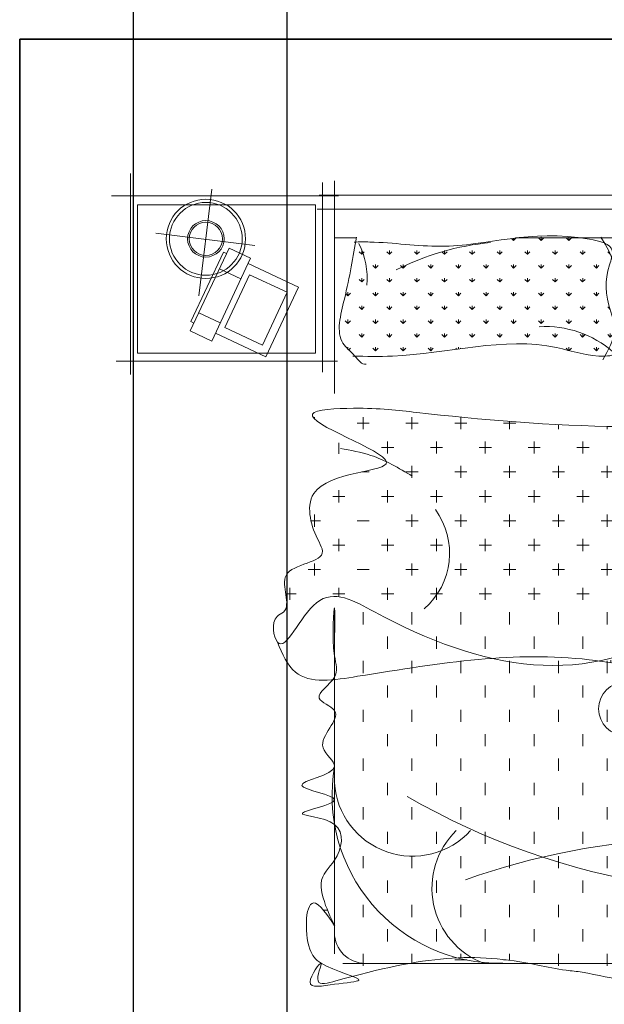
# Model space of a CAD drawing. Units: inches. Extents: x -438 to 102, y -60 to 1091.
# Tile 7 of 20: x -303 to -243, y 699 to 799. Entities that reach past the tile are written whole.
import ezdxf

# ---------------------------------------------------------------- set-up
doc = ezdxf.new("R2010")
doc.units = ezdxf.units.IN
doc.header["$MEASUREMENT"] = 0
doc.layers.add('A-ANNO-DIMS', color=217, linetype='Continuous', lineweight=18, true_color=0x93278f)
doc.layers.add('A-WALL', color=2, linetype='Continuous', lineweight=35, true_color=0xf1eb1f)
doc.layers.add('Furniture', color=7, linetype='Continuous', lineweight=15)
doc.styles.get("Standard").update_dxf_attribs({"font": 'arial.ttf'})
doc.dimstyles.get("Standard").update_dxf_attribs({"dimtxt": 8, "dimasz": 0.18, "dimexe": 0.18, "dimexo": 0.0625, "dimgap": 0.09, "dimtad": 0, "dimtih": 1, "dimtoh": 1, "dimdec": 4, "dimzin": 0, "dimdsep": 46, "dimlunit": 3, "dimtxsty": 'Standard', "dimcen": 0.09, "dimadec": 0, "dimazin": 0, "dimtfac": 1, "dimtdec": 4, "dimtofl": 0, "dimtmove": 0, "dimatfit": 3, "dimfxl": 1, "dimtolj": 1, "dimtzin": 0, "dimarcsym": 0})

# ---------------------------------------------------------------- blocks, each defined once
blk = doc.blocks.new('BED-DOUBLE-WITH-NIGHTSTANDS')
for p, q in [((-50.06, 0), (-50.06, -20.6)), ((30.68, 0), (30.68, -20.6)), ((-30.37, -20.33), (-30.37, -0.9)), ((-29.16, -22.53), (-29.16, -0.74)), ((50.37, -20.33), (50.37, -0.9)), ((-41.72, -1.6), (-43.05, -12.53)), ((29.9, -1.01), (29.9, -27.13)), ((-28.76, -2.28), (-51.98, -2.28)), ((-30.74, -2.19), (29.9, -2.19)), ((51.99, -2.28), (28.76, -2.28)), ((-31.1, -3.21), (-49.32, -3.21)), ((-49.32, -3.21), (-49.32, -18.39)), ((-31.1, -18.39), (-31.1, -3.21)), ((30.68, -3.64), (-30.92, -3.64)), ((49.65, -3.21), (31.43, -3.21)), ((31.43, -3.21), (31.43, -18.39)), ((40.58, -3.96), (40.58, -15.85)), ((49.65, -18.39), (49.65, -3.21)), ((-37.32, -7.35), (-47.47, -6.1)), ((-26.93, -6.59), (-29.16, -6.59)), ((-10.82, -6.85), (-11.02, -6.64)), ((-10.82, -6.85), (-10.55, -6.59)), ((-10.82, -6.85), (-10.82, -6.62)), ((4.24, -6.59), (-10.63, -6.59)), ((-7.99, -6.85), (-8.25, -6.59)), ((-7.99, -6.85), (-7.99, -6.48)), ((-7.99, -6.85), (-7.72, -6.59)), ((-5.16, -6.85), (-5.42, -6.59)), ((-5.16, -6.85), (-5.16, -6.48)), ((-5.16, -6.85), (-4.89, -6.59)), ((5.02, -6.85), (4.75, -6.59)), ((5.02, -6.85), (5.02, -6.53)), ((5.02, -6.85), (5.28, -6.59)), ((29.9, -6.59), (7.41, -6.59)), ((7.85, -6.85), (7.61, -6.61)), ((7.85, -6.85), (7.85, -6.64)), ((7.85, -6.85), (8.03, -6.66)), ((-43.93, -16.11), (-39.96, -7.63)), ((-40.53, -8.03), (-43.86, -15.16)), ((-40.22, -8.18), (-40.53, -8.03)), ((-39.96, -7.63), (-37.75, -8.67)), ((-26.37, -8.26), (-26.64, -8)), ((-26.37, -8.27), (-26.37, -7.89)), ((-26.37, -8.26), (-26.11, -8)), ((-23.54, -8.26), (-23.81, -8)), ((-23.54, -8.27), (-23.54, -7.89)), ((-23.54, -8.26), (-23.28, -8)), ((-20.72, -8.26), (-20.98, -8)), ((-20.72, -8.27), (-20.72, -7.89)), ((-20.72, -8.26), (-20.45, -8)), ((-17.89, -8.26), (-18.15, -8)), ((-17.89, -8.27), (-17.89, -7.89)), ((-17.89, -8.26), (-17.62, -8)), ((-15.06, -8.26), (-15.32, -8)), ((-15.06, -8.27), (-15.06, -7.89)), ((-15.06, -8.26), (-14.79, -8)), ((-12.23, -8.26), (-12.5, -8)), ((-12.23, -8.27), (-12.23, -7.89)), ((-12.23, -8.26), (-11.97, -8)), ((-9.4, -8.26), (-9.67, -8)), ((-9.4, -8.27), (-9.4, -7.89)), ((-9.4, -8.26), (-9.14, -8)), ((-6.57, -8.26), (-6.84, -8)), ((-6.57, -8.27), (-6.57, -7.89)), ((-6.57, -8.26), (-6.31, -8)), ((-3.75, -8.26), (-4.01, -8)), ((-3.75, -8.26), (-3.48, -8)), ((-3.74, -8.27), (-3.74, -7.89)), ((-0.92, -8.26), (-1.18, -8)), ((1.02, -8.02), (1.04, -8)), ((3.6, -8.26), (3.34, -8)), ((3.6, -8.27), (3.6, -7.89)), ((3.6, -8.26), (3.87, -8)), ((6.43, -8.26), (6.17, -8)), ((6.43, -8.27), (6.43, -7.89)), ((6.43, -8.26), (6.7, -8)), ((9.26, -8.26), (9, -8)), ((9.26, -8.27), (9.26, -7.89)), ((9.26, -8.26), (9.53, -8)), ((12.09, -8.26), (11.82, -8)), ((12.09, -8.27), (12.09, -7.89)), ((12.09, -8.26), (12.35, -8)), ((14.92, -8.26), (14.65, -8)), ((14.92, -8.27), (14.92, -7.89)), ((14.92, -8.26), (15.18, -8)), ((17.75, -8.26), (17.48, -8)), ((17.75, -8.27), (17.75, -7.89)), ((17.75, -8.26), (18.01, -8)), ((20.57, -8.26), (20.31, -8)), ((20.57, -8.27), (20.57, -7.89)), ((20.57, -8.26), (20.84, -8)), ((23.4, -8.26), (23.14, -8)), ((23.4, -8.27), (23.4, -7.89)), ((23.4, -8.26), (23.67, -8)), ((26.23, -8.26), (25.97, -8)), ((26.23, -8.27), (26.23, -7.89)), ((26.23, -8.26), (26.5, -8)), ((-37.75, -8.67), (-41.72, -17.15)), ((-0.92, -8.27), (-0.92, -8.26)), ((-0.92, -8.26), (-0.91, -8.26)), ((-38.74, -10.79), (-40.95, -9.75)), ((-32.84, -11.63), (-38.01, -9.21)), ((-24.96, -9.68), (-25.22, -9.41)), ((-24.96, -9.68), (-24.96, -9.3)), ((-24.96, -9.68), (-24.69, -9.41)), ((-22.13, -9.68), (-22.4, -9.41)), ((-22.13, -9.68), (-22.13, -9.3)), ((-22.13, -9.68), (-21.86, -9.41)), ((-19.3, -9.68), (-19.57, -9.41)), ((-19.3, -9.68), (-19.3, -9.3)), ((-19.3, -9.68), (-19.04, -9.41)), ((-16.47, -9.68), (-16.74, -9.41)), ((-16.47, -9.68), (-16.47, -9.3)), ((-16.47, -9.68), (-16.21, -9.41)), ((-13.64, -9.68), (-13.91, -9.41)), ((-13.64, -9.68), (-13.64, -9.3)), ((-13.64, -9.68), (-13.38, -9.41)), ((-10.82, -9.68), (-11.08, -9.41)), ((-10.82, -9.68), (-10.82, -9.3)), ((-10.82, -9.68), (-10.55, -9.41)), ((-7.99, -9.68), (-8.25, -9.41)), ((-7.99, -9.68), (-7.99, -9.3)), ((-7.99, -9.68), (-7.72, -9.41)), ((-5.16, -9.68), (-5.42, -9.41)), ((-5.16, -9.68), (-5.16, -9.3)), ((-5.16, -9.68), (-4.89, -9.41)), ((-2.33, -9.68), (-2.6, -9.41)), ((-2.33, -9.68), (-2.33, -9.3)), ((-2.33, -9.68), (-2.07, -9.41)), ((2.19, -9.68), (1.92, -9.41)), ((2.19, -9.68), (2.19, -9.3)), ((2.19, -9.68), (2.45, -9.41)), ((5.02, -9.68), (4.75, -9.41)), ((5.02, -9.68), (5.02, -9.3)), ((5.02, -9.68), (5.28, -9.41)), ((7.85, -9.68), (7.58, -9.41)), ((7.85, -9.68), (7.85, -9.3)), ((7.85, -9.68), (8.11, -9.41)), ((10.67, -9.68), (10.41, -9.41)), ((10.67, -9.68), (10.94, -9.41)), ((10.68, -9.68), (10.68, -9.3)), ((13.5, -9.68), (13.24, -9.41)), ((13.5, -9.68), (13.5, -9.3)), ((13.5, -9.68), (13.77, -9.41)), ((16.33, -9.68), (16.07, -9.41)), ((16.33, -9.68), (16.33, -9.3)), ((16.33, -9.68), (16.6, -9.41)), ((19.16, -9.68), (18.89, -9.41)), ((19.16, -9.68), (19.16, -9.3)), ((19.16, -9.68), (19.43, -9.41)), ((21.99, -9.68), (21.72, -9.41)), ((21.99, -9.68), (21.99, -9.3)), ((21.99, -9.68), (22.25, -9.41)), ((24.82, -9.68), (24.55, -9.41)), ((24.82, -9.68), (24.82, -9.3)), ((24.82, -9.68), (25.08, -9.41)), ((27.65, -9.68), (27.38, -9.41)), ((27.65, -9.68), (27.65, -9.3)), ((27.65, -9.68), (27.91, -9.41)), ((-37.86, -10.36), (-40.39, -15.77)), ((-34, -12.16), (-37.86, -10.36)), ((-26.37, -11.09), (-26.64, -10.83)), ((-26.37, -11.09), (-26.37, -10.72)), ((-26.37, -11.09), (-26.11, -10.83)), ((-23.54, -11.09), (-23.81, -10.83)), ((-23.54, -11.09), (-23.54, -10.72)), ((-23.54, -11.09), (-23.28, -10.83)), ((-20.72, -11.09), (-20.98, -10.83)), ((-20.72, -11.09), (-20.72, -10.72)), ((-20.72, -11.09), (-20.45, -10.83)), ((-17.89, -11.09), (-18.15, -10.83)), ((-17.89, -11.09), (-17.89, -10.72)), ((-17.89, -11.09), (-17.62, -10.83)), ((-15.06, -11.09), (-15.32, -10.83)), ((-15.06, -11.09), (-15.06, -10.72)), ((-15.06, -11.09), (-14.79, -10.83)), ((-12.23, -11.09), (-12.5, -10.83)), ((-12.23, -11.09), (-12.23, -10.72)), ((-12.23, -11.09), (-11.97, -10.83)), ((-9.4, -11.09), (-9.67, -10.83)), ((-9.4, -11.09), (-9.4, -10.72)), ((-9.4, -11.09), (-9.14, -10.83)), ((-6.57, -11.09), (-6.84, -10.83)), ((-6.57, -11.09), (-6.57, -10.72)), ((-6.57, -11.09), (-6.31, -10.83)), ((-3.75, -11.09), (-4.01, -10.83)), ((-3.75, -11.09), (-3.48, -10.83)), ((-3.74, -11.09), (-3.74, -10.72)), ((3.6, -11.09), (3.34, -10.83)), ((3.6, -11.09), (3.6, -10.72)), ((3.6, -11.09), (3.87, -10.83)), ((6.43, -11.09), (6.17, -10.83)), ((6.43, -11.09), (6.43, -10.72)), ((6.43, -11.09), (6.7, -10.83)), ((9.26, -11.09), (9, -10.83)), ((9.26, -11.09), (9.26, -10.72)), ((9.26, -11.09), (9.53, -10.83)), ((12.09, -11.09), (11.82, -10.83)), ((12.09, -11.09), (12.09, -10.72)), ((12.09, -11.09), (12.35, -10.83)), ((14.92, -11.09), (14.65, -10.83)), ((14.92, -11.09), (14.92, -10.72)), ((14.92, -11.09), (15.18, -10.83)), ((17.75, -11.09), (17.48, -10.83)), ((17.75, -11.09), (17.75, -10.72)), ((17.75, -11.09), (18.01, -10.83)), ((20.57, -11.09), (20.31, -10.83)), ((20.57, -11.09), (20.57, -10.72)), ((20.57, -11.09), (20.84, -10.83)), ((23.4, -11.09), (23.14, -10.83)), ((23.4, -11.09), (23.4, -10.72)), ((23.4, -11.09), (23.67, -10.83)), ((26.23, -11.09), (25.97, -10.83)), ((26.23, -11.09), (26.23, -10.72)), ((26.23, -11.09), (26.5, -10.83)), ((46.48, -10.21), (34.68, -10.21)), ((-36.18, -18.76), (-32.84, -11.63)), ((-36.53, -17.57), (-34, -12.16)), ((-27.79, -12.51), (-28.01, -12.28)), ((-27.79, -12.51), (-27.79, -12.13)), ((-27.79, -12.51), (-27.52, -12.24)), ((-24.96, -12.51), (-25.22, -12.24)), ((-24.96, -12.51), (-24.96, -12.13)), ((-24.96, -12.51), (-24.69, -12.24)), ((-22.13, -12.51), (-22.4, -12.24)), ((-22.13, -12.51), (-22.13, -12.13)), ((-22.13, -12.51), (-21.86, -12.24)), ((-19.3, -12.51), (-19.57, -12.24)), ((-19.3, -12.51), (-19.3, -12.13)), ((-19.3, -12.51), (-19.04, -12.24)), ((-16.47, -12.51), (-16.74, -12.24)), ((-16.47, -12.51), (-16.47, -12.13)), ((-16.47, -12.51), (-16.21, -12.24)), ((-13.64, -12.51), (-13.91, -12.24)), ((-13.64, -12.51), (-13.64, -12.13)), ((-13.64, -12.51), (-13.38, -12.24)), ((-10.82, -12.51), (-11.08, -12.24)), ((-10.82, -12.51), (-10.82, -12.13)), ((-10.82, -12.51), (-10.55, -12.24)), ((-7.99, -12.51), (-8.25, -12.24)), ((-7.99, -12.51), (-7.99, -12.13)), ((-7.99, -12.51), (-7.72, -12.24)), ((-5.16, -12.51), (-5.42, -12.24)), ((-5.16, -12.51), (-5.16, -12.13)), ((-5.16, -12.51), (-4.89, -12.24)), ((-2.33, -12.51), (-2.6, -12.24)), ((-2.33, -12.51), (-2.33, -12.13)), ((-2.33, -12.51), (-2.07, -12.24)), ((2.19, -12.51), (1.92, -12.24)), ((2.19, -12.51), (2.19, -12.13)), ((2.19, -12.51), (2.45, -12.24)), ((5.02, -12.51), (4.75, -12.24)), ((5.02, -12.51), (5.02, -12.13)), ((5.02, -12.51), (5.28, -12.24)), ((7.85, -12.51), (7.58, -12.24)), ((7.85, -12.51), (7.85, -12.13)), ((7.85, -12.51), (8.11, -12.24)), ((10.67, -12.51), (10.41, -12.24)), ((10.67, -12.51), (10.94, -12.24)), ((10.68, -12.51), (10.68, -12.13)), ((13.5, -12.51), (13.24, -12.24)), ((13.5, -12.51), (13.5, -12.13)), ((13.5, -12.51), (13.77, -12.24)), ((16.33, -12.51), (16.07, -12.24)), ((16.33, -12.51), (16.33, -12.13)), ((16.33, -12.51), (16.6, -12.24)), ((19.16, -12.51), (18.89, -12.24)), ((19.16, -12.51), (19.16, -12.13)), ((19.16, -12.51), (19.43, -12.24)), ((21.99, -12.51), (21.72, -12.24)), ((21.99, -12.51), (21.99, -12.13)), ((21.99, -12.51), (22.25, -12.24)), ((24.82, -12.51), (24.55, -12.24)), ((24.82, -12.51), (24.82, -12.13)), ((24.82, -12.51), (25.08, -12.24)), ((27.65, -12.51), (27.38, -12.24)), ((27.65, -12.51), (27.65, -12.13)), ((27.65, -12.51), (27.91, -12.24)), ((-26.37, -13.92), (-26.64, -13.66)), ((-26.37, -13.92), (-26.37, -13.55)), ((-26.37, -13.92), (-26.11, -13.66)), ((-23.54, -13.92), (-23.81, -13.66)), ((-23.54, -13.92), (-23.54, -13.55)), ((-23.54, -13.92), (-23.28, -13.66)), ((-20.72, -13.92), (-20.98, -13.66)), ((-20.72, -13.92), (-20.72, -13.55)), ((-20.72, -13.92), (-20.45, -13.66)), ((-17.89, -13.92), (-18.15, -13.66)), ((-17.89, -13.92), (-17.89, -13.55)), ((-17.89, -13.92), (-17.62, -13.66)), ((-15.06, -13.92), (-15.32, -13.66)), ((-15.06, -13.92), (-15.06, -13.55)), ((-15.06, -13.92), (-14.79, -13.66)), ((-12.23, -13.92), (-12.5, -13.66)), ((-12.23, -13.92), (-12.23, -13.55)), ((-12.23, -13.92), (-11.97, -13.66)), ((-9.4, -13.92), (-9.67, -13.66)), ((-9.4, -13.92), (-9.4, -13.55)), ((-9.4, -13.92), (-9.14, -13.66)), ((-6.57, -13.92), (-6.84, -13.66)), ((-6.57, -13.92), (-6.57, -13.55)), ((-6.57, -13.92), (-6.31, -13.66)), ((-3.75, -13.92), (-4.01, -13.66)), ((-3.75, -13.92), (-3.48, -13.66)), ((-3.74, -13.92), (-3.74, -13.55)), ((-0.93, -13.91), (-1.18, -13.66)), ((1.02, -13.67), (1.04, -13.66)), ((3.6, -13.92), (3.34, -13.66)), ((3.6, -13.92), (3.6, -13.55)), ((3.6, -13.92), (3.87, -13.66)), ((6.43, -13.92), (6.17, -13.66)), ((6.43, -13.92), (6.43, -13.55)), ((6.43, -13.92), (6.7, -13.66)), ((9.26, -13.92), (9, -13.66)), ((9.26, -13.92), (9.26, -13.55)), ((9.26, -13.92), (9.53, -13.66)), ((12.09, -13.92), (11.82, -13.66)), ((12.09, -13.92), (12.09, -13.55)), ((12.09, -13.92), (12.35, -13.66)), ((14.92, -13.92), (14.65, -13.66)), ((14.92, -13.92), (14.92, -13.55)), ((14.92, -13.92), (15.18, -13.66)), ((17.75, -13.92), (17.48, -13.66)), ((17.75, -13.92), (17.75, -13.55)), ((17.75, -13.92), (18.01, -13.66)), ((20.57, -13.92), (20.31, -13.66)), ((20.57, -13.92), (20.57, -13.55)), ((20.57, -13.92), (20.84, -13.66)), ((23.4, -13.92), (23.14, -13.66)), ((23.4, -13.92), (23.4, -13.55)), ((23.4, -13.92), (23.67, -13.66)), ((26.23, -13.92), (25.97, -13.66)), ((26.23, -13.92), (26.23, -13.55)), ((26.23, -13.92), (26.5, -13.66)), ((-40.85, -15.29), (-43.06, -14.25)), ((-27.79, -15.34), (-28.05, -15.07)), ((-27.79, -15.34), (-27.79, -14.96)), ((-27.79, -15.34), (-27.52, -15.07)), ((-24.96, -15.34), (-25.22, -15.07)), ((-24.96, -15.34), (-24.96, -14.96)), ((-24.96, -15.34), (-24.69, -15.07)), ((-22.13, -15.34), (-22.4, -15.07)), ((-22.13, -15.34), (-22.13, -14.96)), ((-22.13, -15.34), (-21.86, -15.07)), ((-19.3, -15.34), (-19.57, -15.07)), ((-19.3, -15.34), (-19.3, -14.96)), ((-19.3, -15.34), (-19.04, -15.07)), ((-16.47, -15.34), (-16.74, -15.07)), ((-16.47, -15.34), (-16.47, -14.96)), ((-16.47, -15.34), (-16.21, -15.07)), ((-13.64, -15.34), (-13.91, -15.07)), ((-13.64, -15.34), (-13.64, -14.96)), ((-13.64, -15.34), (-13.38, -15.07)), ((-10.82, -15.34), (-11.08, -15.07)), ((-10.82, -15.34), (-10.82, -14.96)), ((-10.82, -15.34), (-10.55, -15.07)), ((-7.99, -15.34), (-8.25, -15.07)), ((-7.99, -15.34), (-7.99, -14.96)), ((-7.99, -15.34), (-7.72, -15.07)), ((-5.16, -15.34), (-5.42, -15.07)), ((-5.16, -15.34), (-5.16, -14.96)), ((-5.16, -15.34), (-4.89, -15.07)), ((-2.33, -15.34), (-2.6, -15.07)), ((-2.33, -15.34), (-2.33, -14.96)), ((-2.33, -15.34), (-2.07, -15.07)), ((2.19, -15.34), (1.92, -15.07)), ((2.19, -15.34), (2.19, -14.96)), ((2.19, -15.34), (2.45, -15.07)), ((5.02, -15.34), (4.75, -15.07)), ((5.02, -15.34), (5.02, -14.96)), ((5.02, -15.34), (5.28, -15.07)), ((7.85, -15.34), (7.58, -15.07)), ((7.85, -15.34), (7.85, -14.96)), ((7.85, -15.34), (8.11, -15.07)), ((10.67, -15.34), (10.41, -15.07)), ((10.67, -15.34), (10.94, -15.07)), ((10.68, -15.34), (10.68, -14.96)), ((13.5, -15.34), (13.24, -15.07)), ((13.5, -15.34), (13.5, -14.96)), ((13.5, -15.34), (13.77, -15.07)), ((16.33, -15.34), (16.07, -15.07)), ((16.33, -15.34), (16.33, -14.96)), ((16.33, -15.34), (16.6, -15.07)), ((19.16, -15.34), (18.89, -15.07)), ((19.16, -15.34), (19.16, -14.96)), ((19.16, -15.34), (19.43, -15.07)), ((21.99, -15.34), (21.72, -15.07)), ((21.99, -15.34), (21.99, -14.96)), ((21.99, -15.34), (22.25, -15.07)), ((24.82, -15.34), (24.55, -15.07)), ((24.82, -15.34), (24.82, -14.96)), ((24.82, -15.34), (25.08, -15.07)), ((27.65, -15.34), (27.38, -15.07)), ((27.65, -15.34), (27.65, -14.96)), ((27.65, -15.34), (27.91, -15.07)), ((-41.72, -17.15), (-43.93, -16.11)), ((-43.86, -15.16), (-43.55, -15.31)), ((-40.39, -15.77), (-36.53, -17.57)), ((-41.34, -16.34), (-36.18, -18.76)), ((-26.37, -16.75), (-26.64, -16.48)), ((-26.37, -16.75), (-26.37, -16.38)), ((-26.37, -16.75), (-26.11, -16.48)), ((-23.54, -16.75), (-23.81, -16.48)), ((-23.54, -16.75), (-23.54, -16.38)), ((-23.54, -16.75), (-23.28, -16.48)), ((-20.72, -16.75), (-20.98, -16.48)), ((-20.72, -16.75), (-20.72, -16.38)), ((-20.72, -16.75), (-20.45, -16.48)), ((-17.89, -16.75), (-18.15, -16.48)), ((-17.89, -16.75), (-17.89, -16.38)), ((-17.89, -16.75), (-17.62, -16.48)), ((-15.06, -16.75), (-15.32, -16.48)), ((-15.06, -16.75), (-15.06, -16.38)), ((-15.06, -16.75), (-14.79, -16.48)), ((-12.23, -16.75), (-12.5, -16.48)), ((-12.23, -16.75), (-12.23, -16.38)), ((-12.23, -16.75), (-11.97, -16.48)), ((-9.4, -16.75), (-9.67, -16.48)), ((-9.4, -16.75), (-9.4, -16.38)), ((-9.4, -16.75), (-9.14, -16.48)), ((-6.57, -16.75), (-6.84, -16.48)), ((-6.57, -16.75), (-6.57, -16.38)), ((-6.57, -16.75), (-6.31, -16.48)), ((-3.75, -16.75), (-4.01, -16.48)), ((-3.75, -16.75), (-3.48, -16.48)), ((-3.74, -16.75), (-3.74, -16.38)), ((-0.92, -16.75), (-1.18, -16.48)), ((-0.92, -16.75), (-0.92, -16.38)), ((-0.92, -16.75), (-0.65, -16.48)), ((0.78, -16.75), (0.51, -16.48)), ((0.78, -16.75), (0.78, -16.38)), ((0.78, -16.75), (1.04, -16.48)), ((3.6, -16.75), (3.34, -16.48)), ((3.6, -16.75), (3.6, -16.38)), ((3.6, -16.75), (3.87, -16.48)), ((6.43, -16.75), (6.17, -16.48)), ((6.43, -16.75), (6.43, -16.38)), ((6.43, -16.75), (6.7, -16.48)), ((9.26, -16.75), (9, -16.48)), ((9.26, -16.75), (9.26, -16.38)), ((9.26, -16.75), (9.53, -16.48)), ((12.09, -16.75), (11.82, -16.48)), ((12.09, -16.75), (12.09, -16.38)), ((12.09, -16.75), (12.35, -16.48)), ((14.92, -16.75), (14.65, -16.48)), ((14.92, -16.75), (14.92, -16.38)), ((14.92, -16.75), (15.18, -16.48)), ((17.75, -16.75), (17.48, -16.48)), ((17.75, -16.75), (17.75, -16.38)), ((17.75, -16.75), (18.01, -16.48)), ((20.57, -16.75), (20.31, -16.48)), ((20.57, -16.75), (20.57, -16.38)), ((20.57, -16.75), (20.84, -16.48)), ((23.4, -16.75), (23.14, -16.48)), ((23.4, -16.75), (23.4, -16.38)), ((23.4, -16.75), (23.67, -16.48)), ((26.23, -16.75), (25.97, -16.48)), ((26.23, -16.75), (26.23, -16.38)), ((26.23, -16.75), (26.5, -16.48)), ((29.06, -16.75), (28.79, -16.48)), ((29.06, -16.75), (29.06, -16.38)), ((29.06, -16.75), (29.27, -16.54)), ((-27.79, -17.97), (-27.79, -17.79)), ((-27.69, -18.07), (-27.52, -17.9)), ((-24.96, -18.16), (-25.22, -17.9)), ((-24.96, -18.16), (-24.96, -17.79)), ((-24.96, -18.16), (-24.69, -17.9)), ((-22.13, -18.16), (-22.4, -17.9)), ((-22.13, -18.16), (-22.13, -17.79)), ((-22.13, -18.16), (-21.86, -17.9)), ((-19.3, -18.16), (-19.57, -17.9)), ((-19.3, -18.16), (-19.3, -17.79)), ((-19.3, -18.16), (-19.04, -17.9)), ((-16.65, -17.99), (-16.74, -17.9)), ((-16.47, -17.96), (-16.47, -17.79)), ((-16.24, -17.93), (-16.21, -17.9)), ((-5.21, -18.11), (-5.42, -17.9)), ((-5.16, -18.13), (-5.16, -17.79)), ((-5.13, -18.13), (-4.89, -17.9)), ((-2.33, -18.16), (-2.6, -17.9)), ((-2.33, -18.16), (-2.33, -17.79)), ((-2.33, -18.16), (-2.07, -17.9)), ((2.19, -18.16), (1.92, -17.9)), ((2.19, -18.16), (2.19, -17.79)), ((2.19, -18.16), (2.45, -17.9)), ((5.02, -18.16), (4.75, -17.9)), ((5.02, -18.16), (5.02, -17.79)), ((5.02, -18.16), (5.28, -17.9)), ((7.85, -18.16), (7.58, -17.9)), ((7.85, -18.16), (7.85, -17.79)), ((7.85, -18.16), (8.11, -17.9)), ((10.68, -17.83), (10.68, -17.79)), ((13.5, -17.88), (13.5, -17.79)), ((13.76, -17.91), (13.77, -17.9)), ((16.33, -18.16), (16.07, -17.9)), ((16.33, -18.16), (16.33, -17.79)), ((16.33, -18.16), (16.6, -17.9)), ((19.16, -18.16), (18.89, -17.9)), ((19.16, -18.16), (19.16, -17.79)), ((19.16, -18.16), (19.43, -17.9)), ((21.99, -18.16), (21.72, -17.9)), ((21.99, -18.16), (21.99, -17.79)), ((21.99, -18.16), (22.25, -17.9)), ((24.82, -18.16), (24.55, -17.9)), ((24.82, -18.16), (24.82, -17.79)), ((24.82, -18.16), (25.08, -17.9)), ((27.65, -18.16), (27.38, -17.9)), ((27.65, -18.16), (27.65, -17.79)), ((27.65, -18.16), (27.91, -17.9)), ((30.17, -21.62), (30.17, -17.94)), ((-49.32, -18.39), (-31.1, -18.39)), ((31.43, -18.39), (49.65, -18.39)), ((-51.53, -19.21), (-28.85, -19.21)), ((3.6, -19.24), (3.6, -19.2)), ((29.21, -19.21), (51.9, -19.21)), ((26.28, -23.69), (26.28, -23.21)), ((-31.22, -25.15), (-31.22, -24.94)), ((-26.22, -26.19), (-26.22, -24.94)), ((-21.22, -26.19), (-21.22, -24.94)), ((-16.22, -26.19), (-16.22, -24.95)), ((13.78, -26.19), (13.78, -25.14)), ((18.78, -26.19), (18.78, -24.94)), ((23.78, -26.19), (23.78, -24.94)), ((28.78, -26.19), (28.78, -24.94)), ((-30.59, -25.57), (-30.67, -25.57)), ((-25.59, -25.57), (-26.84, -25.57)), ((-20.59, -25.57), (-21.84, -25.57)), ((-15.59, -25.57), (-16.84, -25.57)), ((-10.59, -25.57), (-11.84, -25.57)), ((-11.22, -26.19), (-11.22, -25.39)), ((-6.22, -26.19), (-6.22, -25.72)), ((-1.22, -26.19), (-1.22, -25.9)), ((3.78, -26.19), (3.78, -25.87)), ((8.78, -26.19), (8.78, -25.62)), ((14.41, -25.57), (13.16, -25.57)), ((19.41, -25.57), (18.16, -25.57)), ((24.41, -25.57), (23.16, -25.57)), ((29.41, -25.57), (28.16, -25.57)), ((-28.71, -28.72), (-28.71, -27.6)), ((-23.09, -28.07), (-24.34, -28.07)), ((-23.72, -28.69), (-23.72, -27.44)), ((-18.09, -28.07), (-19.34, -28.07)), ((-18.72, -28.69), (-18.72, -27.44)), ((-13.09, -28.07), (-14.34, -28.07)), ((-13.72, -28.69), (-13.72, -27.44)), ((-8.09, -28.07), (-9.34, -28.07)), ((-8.72, -28.69), (-8.72, -27.44)), ((-3.09, -28.07), (-4.34, -28.07)), ((-3.72, -28.69), (-3.72, -27.44)), ((1.91, -28.07), (0.66, -28.07)), ((1.28, -28.69), (1.28, -27.44)), ((6.91, -28.07), (5.66, -28.07)), ((6.28, -28.69), (6.28, -27.44)), ((11.91, -28.07), (10.66, -28.07)), ((11.28, -28.69), (11.28, -27.44)), ((16.91, -28.07), (15.66, -28.07)), ((16.28, -28.69), (16.28, -27.44)), ((21.91, -28.07), (20.66, -28.07)), ((21.28, -28.69), (21.28, -27.44)), ((26.91, -28.07), (25.66, -28.07)), ((26.28, -28.69), (26.28, -27.44)), ((31.91, -28.07), (30.66, -28.07)), ((31.28, -28.69), (31.28, -27.44)), ((-21.22, -31.19), (-21.22, -29.94)), ((-16.22, -31.19), (-16.22, -29.94)), ((-11.22, -31.19), (-11.22, -29.94)), ((-6.22, -31.19), (-6.22, -29.94)), ((-1.22, -31.19), (-1.22, -29.94)), ((3.78, -31.19), (3.78, -29.94)), ((8.78, -31.19), (8.78, -29.94)), ((13.78, -31.19), (13.78, -29.94)), ((18.78, -31.19), (18.78, -29.94)), ((23.78, -31.19), (23.78, -29.94)), ((28.78, -31.19), (28.78, -29.94)), ((-25.59, -30.57), (-26.37, -30.57)), ((-20.59, -30.57), (-21.84, -30.57)), ((-15.59, -30.57), (-16.84, -30.57)), ((-10.59, -30.57), (-11.84, -30.57)), ((-5.59, -30.57), (-6.84, -30.57)), ((-0.59, -30.57), (-1.84, -30.57)), ((4.41, -30.57), (3.16, -30.57)), ((9.41, -30.57), (8.16, -30.57)), ((14.41, -30.57), (13.16, -30.57)), ((19.41, -30.57), (18.16, -30.57)), ((24.41, -30.57), (23.16, -30.57)), ((29.41, -30.57), (28.16, -30.57)), ((-28.09, -33.07), (-29.34, -33.07)), ((-28.72, -33.69), (-28.72, -32.44)), ((-23.09, -33.07), (-24.34, -33.07)), ((-23.72, -33.69), (-23.72, -32.44)), ((-18.09, -33.07), (-19.34, -33.07)), ((-18.72, -33.69), (-18.72, -32.44)), ((-13.09, -33.07), (-14.34, -33.07)), ((-13.72, -33.69), (-13.72, -32.44)), ((-8.09, -33.07), (-9.34, -33.07)), ((-8.72, -33.69), (-8.72, -32.44)), ((-3.09, -33.07), (-4.34, -33.07)), ((-3.72, -33.69), (-3.72, -32.44)), ((1.91, -33.07), (0.66, -33.07)), ((1.28, -33.69), (1.28, -32.44)), ((6.91, -33.07), (5.66, -33.07)), ((6.28, -33.69), (6.28, -32.44)), ((11.91, -33.07), (10.66, -33.07)), ((11.28, -33.69), (11.28, -32.44)), ((16.91, -33.07), (15.66, -33.07)), ((16.28, -33.69), (16.28, -32.44)), ((21.91, -33.07), (20.66, -33.07)), ((21.28, -33.69), (21.28, -32.44)), ((26.91, -33.07), (25.66, -33.07)), ((26.28, -33.69), (26.28, -32.44)), ((31.91, -33.07), (30.66, -33.07)), ((31.28, -33.69), (31.28, -32.44)), ((-31.22, -36.19), (-31.22, -34.94)), ((-21.22, -36.19), (-21.22, -34.94)), ((-16.22, -36.19), (-16.22, -34.94)), ((-11.22, -36.19), (-11.22, -34.94)), ((-6.22, -36.19), (-6.22, -34.94)), ((-1.22, -36.19), (-1.22, -34.94)), ((3.78, -36.19), (3.78, -34.94)), ((13.78, -36.19), (13.78, -34.94)), ((18.78, -36.19), (18.78, -34.94)), ((23.78, -36.19), (23.78, -34.94)), ((28.78, -36.19), (28.78, -34.94)), ((-30.59, -35.57), (-31.57, -35.57)), ((-25.59, -35.57), (-26.84, -35.57)), ((-20.59, -35.57), (-21.84, -35.57)), ((-15.59, -35.57), (-16.84, -35.57)), ((-10.59, -35.57), (-11.84, -35.57)), ((-5.59, -35.57), (-6.84, -35.57)), ((-0.59, -35.57), (-1.84, -35.57)), ((4.41, -35.57), (3.16, -35.57)), ((14.41, -35.57), (13.16, -35.57)), ((19.41, -35.57), (18.16, -35.57)), ((24.41, -35.57), (23.16, -35.57)), ((29.41, -35.57), (28.16, -35.57)), ((-28.09, -38.07), (-29.34, -38.07)), ((-28.72, -38.69), (-28.72, -37.44)), ((-23.09, -38.07), (-24.34, -38.07)), ((-23.72, -38.69), (-23.72, -37.44)), ((-18.09, -38.07), (-19.34, -38.07)), ((-18.72, -38.69), (-18.72, -37.44)), ((-13.09, -38.07), (-14.34, -38.07)), ((-13.72, -38.69), (-13.72, -37.44)), ((-8.09, -38.07), (-9.34, -38.07)), ((-8.72, -38.69), (-8.72, -37.44)), ((-3.09, -38.07), (-4.34, -38.07)), ((-3.72, -38.69), (-3.72, -37.44)), ((1.91, -38.07), (0.66, -38.07)), ((1.28, -38.69), (1.28, -37.44)), ((6.91, -38.07), (5.66, -38.07)), ((11.91, -38.07), (10.66, -38.07)), ((11.28, -38.69), (11.28, -37.44)), ((16.91, -38.07), (15.66, -38.07)), ((16.28, -38.69), (16.28, -37.44)), ((21.91, -38.07), (20.66, -38.07)), ((21.28, -38.69), (21.28, -37.44)), ((26.91, -38.07), (25.66, -38.07)), ((26.28, -38.69), (26.28, -37.44)), ((31.91, -38.07), (30.66, -38.07)), ((31.28, -38.69), (31.28, -37.44)), ((-31.22, -41.19), (-31.22, -39.94)), ((-21.22, -41.19), (-21.22, -39.94)), ((-16.22, -41.19), (-16.22, -39.94)), ((-11.22, -41.19), (-11.22, -39.94)), ((-6.22, -41.19), (-6.22, -39.94)), ((-1.22, -41.19), (-1.22, -39.94)), ((3.78, -41.19), (3.78, -39.94)), ((13.78, -41.19), (13.78, -39.94)), ((18.78, -41.19), (18.78, -39.94)), ((23.78, -41.19), (23.78, -39.94)), ((28.78, -41.19), (28.78, -39.94)), ((33.78, -41.19), (33.78, -39.94)), ((-30.59, -40.57), (-31.84, -40.57)), ((-25.59, -40.57), (-26.84, -40.57)), ((-20.59, -40.57), (-21.84, -40.57)), ((-15.59, -40.57), (-16.84, -40.57)), ((-10.59, -40.57), (-11.84, -40.57)), ((-5.59, -40.57), (-6.84, -40.57)), ((-0.59, -40.57), (-1.84, -40.57)), ((4.41, -40.57), (3.16, -40.57)), ((9.41, -40.57), (8.16, -40.57)), ((14.1, -40.57), (13.16, -40.57)), ((20.16, -40.97), (19.43, -40.97)), ((19.79, -41.34), (19.79, -40.86)), ((24.41, -40.57), (24.09, -40.57)), ((29.41, -40.57), (28.16, -40.57)), ((29.9, -41), (29.9, -83.36)), ((34.41, -40.57), (33.16, -40.57)), ((18.32, -42.82), (18.32, -42.08)), ((21.27, -42.82), (21.27, -42.08)), ((24.22, -42.82), (24.22, -42.22)), ((-33.09, -43.07), (-34.15, -43.07)), ((-33.72, -43.69), (-33.72, -42.44)), ((-28.09, -43.07), (-29.34, -43.07)), ((-28.72, -43.37), (-28.72, -42.44)), ((-23.09, -43.07), (-24.34, -43.07)), ((-23.72, -43.69), (-23.72, -42.44)), ((-18.09, -43.07), (-19.34, -43.07)), ((-18.72, -43.69), (-18.72, -42.44)), ((-13.09, -43.07), (-14.34, -43.07)), ((-13.72, -43.69), (-13.72, -42.44)), ((-8.09, -43.07), (-9.34, -43.07)), ((-8.72, -43.69), (-8.72, -42.44)), ((-3.09, -43.07), (-4.34, -43.07)), ((-3.72, -43.69), (-3.72, -42.44)), ((1.91, -43.07), (0.66, -43.07)), ((1.28, -43.69), (1.28, -42.44)), ((6.91, -43.07), (5.66, -43.07)), ((10.92, -43.07), (10.66, -43.07)), ((11.28, -43.69), (11.28, -42.44)), ((15.37, -42.82), (15.37, -42.52)), ((15.73, -42.45), (15.5, -42.45)), ((16.28, -43.69), (16.28, -42.44)), ((18.69, -42.45), (17.95, -42.45)), ((21.64, -42.45), (20.9, -42.45)), ((21.28, -43.69), (21.28, -42.44)), ((24.59, -42.45), (23.85, -42.45)), ((26.28, -43.69), (26.28, -42.44)), ((31.91, -43.07), (30.66, -43.07)), ((31.28, -43.69), (31.28, -42.44)), ((14.26, -43.92), (13.52, -43.92)), ((13.89, -44.29), (13.89, -43.56)), ((17.21, -43.92), (16.47, -43.92)), ((16.84, -44.29), (16.84, -43.56)), ((20.16, -43.92), (19.43, -43.92)), ((19.79, -44.29), (19.79, -43.56)), ((23.12, -43.92), (22.38, -43.92)), ((22.75, -44.29), (22.75, -43.56)), ((26.07, -43.92), (25.33, -43.92)), ((25.7, -44.29), (25.7, -43.56)), ((-29.16, -79.94), (-29.16, -44.49)), ((-26.22, -46.19), (-26.22, -44.94)), ((-21.22, -46.19), (-21.22, -44.94)), ((-16.22, -46.19), (-16.22, -44.94)), ((-11.22, -46.19), (-11.22, -44.94)), ((-6.22, -46.19), (-6.22, -44.94)), ((-1.22, -46.19), (-1.22, -44.94)), ((3.78, -46.19), (3.78, -44.94)), ((8.78, -46.19), (8.78, -44.94)), ((12.78, -45.4), (12.04, -45.4)), ((12.41, -45.77), (12.41, -45.03)), ((13.78, -46.19), (13.78, -44.94)), ((15.73, -45.4), (15, -45.4)), ((15.37, -45.77), (15.37, -45.03)), ((18.69, -45.4), (17.95, -45.4)), ((18.32, -45.77), (18.32, -45.03)), ((18.78, -46.19), (18.78, -44.94)), ((21.64, -45.4), (20.9, -45.4)), ((21.27, -45.77), (21.27, -45.03)), ((23.78, -46.19), (23.78, -44.94)), ((24.47, -45.4), (23.85, -45.4)), ((24.22, -45.56), (24.22, -45.03)), ((28.78, -46.19), (28.78, -44.94)), ((9.41, -45.57), (8.16, -45.57)), ((14.41, -45.57), (13.16, -45.57)), ((19.41, -45.57), (18.16, -45.57)), ((24.41, -45.57), (23.16, -45.57)), ((29.41, -45.57), (28.16, -45.57)), ((7.98, -47.25), (7.98, -47.2)), ((11.31, -46.88), (10.57, -46.88)), ((10.94, -47.25), (10.94, -46.51)), ((14.26, -46.88), (13.52, -46.88)), ((13.89, -47.25), (13.89, -46.51)), ((17.21, -46.88), (16.47, -46.88)), ((16.84, -47.25), (16.84, -46.51)), ((20.16, -46.88), (19.43, -46.88)), ((19.79, -47.25), (19.79, -46.51)), ((22.55, -46.88), (22.38, -46.88)), ((22.75, -46.7), (22.75, -46.51)), ((-34.33, -48.07), (-34.34, -48.07)), ((-23.72, -48.69), (-23.72, -47.44)), ((-18.72, -48.69), (-18.72, -47.44)), ((-13.72, -48.69), (-13.72, -47.44)), ((-8.72, -48.69), (-8.72, -47.44)), ((-3.72, -48.69), (-3.72, -47.44)), ((1.28, -48.69), (1.28, -47.44)), ((6.91, -48.07), (5.66, -48.07)), ((6.88, -48.35), (6.14, -48.35)), ((6.28, -48.69), (6.28, -47.44)), ((6.51, -48.72), (6.51, -47.98)), ((9.83, -48.35), (9.09, -48.35)), ((9.46, -48.72), (9.46, -47.98)), ((11.91, -48.07), (10.66, -48.07)), ((11.28, -48.69), (11.28, -47.44)), ((12.78, -48.35), (12.04, -48.35)), ((12.41, -48.72), (12.41, -47.98)), ((15.73, -48.35), (15, -48.35)), ((15.37, -48.72), (15.37, -47.98)), ((16.91, -48.07), (15.66, -48.07)), ((16.28, -48.69), (16.28, -47.44)), ((18.69, -48.35), (17.95, -48.35)), ((18.32, -48.72), (18.32, -47.98)), ((21.91, -48.07), (20.66, -48.07)), ((21.02, -48.35), (20.9, -48.35)), ((21.27, -48.11), (21.27, -47.98)), ((21.28, -48.69), (21.28, -47.44)), ((26.91, -48.07), (25.66, -48.07)), ((26.28, -48.69), (26.28, -47.44)), ((-26.22, -51.19), (-26.22, -49.94)), ((-21.22, -51.19), (-21.22, -49.94)), ((-16.22, -51.19), (-16.22, -49.94)), ((-11.22, -51.19), (-11.22, -49.94)), ((-6.22, -51.19), (-6.22, -49.94)), ((-1.22, -51.19), (-1.22, -49.94)), ((-0.87, -50.11), (-0.87, -49.87)), ((2.45, -49.83), (1.71, -49.83)), ((2.08, -50.2), (2.08, -49.46)), ((3.78, -51.19), (3.78, -49.94)), ((5.4, -49.83), (4.66, -49.83)), ((5.03, -50.2), (5.03, -49.46)), ((8.35, -49.83), (7.61, -49.83)), ((7.98, -50.2), (7.98, -49.46)), ((8.78, -51.19), (8.78, -49.94)), ((11.31, -49.83), (10.57, -49.83)), ((10.94, -50.2), (10.94, -49.46)), ((14.26, -49.83), (13.52, -49.83)), ((13.78, -51.19), (13.78, -49.94)), ((13.89, -50.2), (13.89, -49.46)), ((17.21, -49.83), (16.47, -49.83)), ((16.84, -50.2), (16.84, -49.46)), ((18.78, -51.19), (18.78, -49.94)), ((19.48, -49.83), (19.43, -49.83)), ((19.79, -49.55), (19.79, -49.46)), ((23.78, -51.19), (23.78, -49.94)), ((28.78, -51.19), (28.78, -49.94)), ((3.55, -50.99), (3.55, -50.94)), ((6.88, -51.31), (6.14, -51.31)), ((6.51, -51.61), (6.51, -50.94)), ((9.83, -51.31), (9.09, -51.31)), ((9.46, -51.68), (9.46, -50.94)), ((12.78, -51.31), (12.04, -51.31)), ((12.41, -51.68), (12.41, -50.94)), ((15.73, -51.31), (15, -51.31)), ((15.37, -51.68), (15.37, -50.94)), ((-23.72, -53.69), (-23.72, -52.44)), ((-18.72, -53.69), (-18.72, -52.44)), ((-13.72, -53.69), (-13.72, -52.44)), ((-8.72, -53.69), (-8.72, -52.44)), ((-3.72, -53.69), (-3.72, -52.44)), ((1.28, -53.69), (1.28, -52.44)), ((6.28, -53.69), (6.28, -52.44)), ((11.28, -53.69), (11.28, -52.44)), ((16.28, -53.69), (16.28, -52.44)), ((21.28, -53.69), (21.28, -52.44)), ((26.28, -53.69), (26.28, -52.44)), ((31.28, -53.69), (31.28, -53.25)), ((-26.22, -56.19), (-26.22, -54.94)), ((-21.22, -56.19), (-21.22, -54.94)), ((-16.22, -56.19), (-16.22, -54.94)), ((-11.22, -56.19), (-11.22, -54.94)), ((-6.22, -56.19), (-6.22, -54.94)), ((-1.22, -56.19), (-1.22, -54.94)), ((3.78, -56.19), (3.78, -54.94)), ((8.78, -56.19), (8.78, -54.94)), ((13.78, -56.19), (13.78, -54.94)), ((18.78, -56.19), (18.78, -54.94)), ((23.78, -56.19), (23.78, -54.94)), ((28.78, -56.19), (28.78, -54.94)), ((-23.72, -58.69), (-23.72, -57.44)), ((-18.72, -58.69), (-18.72, -57.44)), ((-13.72, -58.69), (-13.72, -57.44)), ((-8.72, -58.69), (-8.72, -57.44)), ((-3.72, -58.69), (-3.72, -57.44)), ((1.28, -58.69), (1.28, -57.44)), ((6.28, -58.69), (6.28, -57.44)), ((11.28, -58.69), (11.28, -57.44)), ((16.28, -58.69), (16.28, -57.44)), ((21.28, -58.69), (21.28, -57.44)), ((26.28, -58.69), (26.28, -57.44)), ((-26.22, -61.19), (-26.22, -59.94)), ((-21.22, -61.19), (-21.22, -59.94)), ((-16.22, -61.19), (-16.22, -59.94)), ((-11.22, -61.19), (-11.22, -59.94)), ((-6.22, -61.19), (-6.22, -59.94)), ((-1.22, -61.19), (-1.22, -59.94)), ((3.78, -61.19), (3.78, -59.94)), ((8.78, -61.19), (8.78, -59.94)), ((13.78, -61.19), (13.78, -59.94)), ((18.78, -61.19), (18.78, -59.94)), ((23.78, -61.19), (23.78, -59.94)), ((28.78, -61.19), (28.78, -59.94)), ((-23.72, -63.69), (-23.72, -62.44)), ((-18.72, -63.69), (-18.72, -62.44)), ((-13.72, -63.69), (-13.72, -62.44)), ((-8.72, -63.69), (-8.72, -62.44)), ((-3.72, -63.69), (-3.72, -62.44)), ((1.28, -63.69), (1.28, -62.44)), ((6.28, -63.69), (6.28, -62.44)), ((11.28, -63.69), (11.28, -62.44)), ((16.28, -63.69), (16.28, -62.44)), ((21.28, -63.69), (21.28, -62.44)), ((26.28, -63.69), (26.28, -62.44)), ((-26.22, -66.19), (-26.22, -64.94)), ((-21.22, -66.19), (-21.22, -64.94)), ((-16.22, -66.19), (-16.22, -64.94)), ((-11.22, -66.19), (-11.22, -64.94)), ((-6.22, -66.19), (-6.22, -64.94)), ((-1.22, -66.19), (-1.22, -64.94)), ((3.78, -66.19), (3.78, -64.94)), ((8.78, -66.19), (8.78, -64.94)), ((13.78, -66.19), (13.78, -64.94)), ((18.78, -66.19), (18.78, -64.94)), ((23.78, -66.19), (23.78, -64.94)), ((28.78, -66.19), (28.78, -64.94)), ((-23.72, -68.69), (-23.72, -67.44)), ((-18.72, -68.69), (-18.72, -67.44)), ((-13.72, -68.69), (-13.72, -67.44)), ((-8.72, -68.69), (-8.72, -67.44)), ((-3.72, -68.69), (-3.72, -67.44)), ((1.28, -68.69), (1.28, -67.44)), ((6.28, -68.69), (6.28, -67.44)), ((11.28, -68.69), (11.28, -67.44)), ((16.28, -68.69), (16.28, -67.44)), ((21.28, -68.69), (21.28, -67.44)), ((26.28, -68.69), (26.28, -67.44)), ((31.28, -68.1), (31.28, -67.44)), ((-26.22, -71.19), (-26.22, -69.94)), ((-21.22, -71.19), (-21.22, -69.94)), ((-16.22, -71.19), (-16.22, -69.94)), ((-11.22, -71.19), (-11.22, -69.94)), ((-6.22, -71.19), (-6.22, -69.94)), ((-1.22, -71.19), (-1.22, -69.94)), ((3.78, -71.19), (3.78, -69.94)), ((8.78, -71.19), (8.78, -69.94)), ((13.78, -71.19), (13.78, -69.94)), ((18.78, -71.19), (18.78, -69.94)), ((23.78, -71.19), (23.78, -69.94)), ((28.78, -71.19), (28.78, -69.94)), ((-23.72, -73.69), (-23.72, -72.44)), ((-18.72, -73.69), (-18.72, -72.44)), ((-13.72, -73.69), (-13.72, -72.44)), ((-8.72, -73.69), (-8.72, -72.44)), ((-3.72, -73.69), (-3.72, -72.44)), ((1.28, -73.69), (1.28, -72.44)), ((6.28, -73.69), (6.28, -72.44)), ((11.28, -73.69), (11.28, -72.44)), ((16.28, -73.69), (16.28, -72.44)), ((21.28, -73.69), (21.28, -72.44)), ((26.28, -73.69), (26.28, -72.44)), ((31.28, -73.69), (31.28, -73.16)), ((-29.87, -75.49), (-30.28, -75.49)), ((-26.22, -76.19), (-26.22, -74.94)), ((-21.22, -76.19), (-21.22, -74.94)), ((-16.22, -76.19), (-16.22, -74.94)), ((-11.22, -76.19), (-11.22, -74.94)), ((-6.22, -76.19), (-6.22, -74.94)), ((-1.22, -76.19), (-1.22, -74.94)), ((3.78, -76.19), (3.78, -74.94)), ((8.78, -76.19), (8.78, -74.94)), ((13.78, -76.19), (13.78, -74.94)), ((18.78, -76.19), (18.78, -74.94)), ((23.78, -76.19), (23.78, -74.94)), ((28.78, -76.19), (28.78, -74.94)), ((-23.72, -78.69), (-23.72, -77.44)), ((-18.72, -78.69), (-18.72, -77.44)), ((-13.72, -78.69), (-13.72, -77.44)), ((-8.72, -78.69), (-8.72, -77.44)), ((-3.72, -78.69), (-3.72, -77.44)), ((1.28, -78.69), (1.28, -77.44)), ((6.28, -78.69), (6.28, -77.44)), ((11.28, -78.69), (11.28, -77.44)), ((16.28, -78.69), (16.28, -77.44)), ((21.28, -78.69), (21.28, -77.44)), ((26.28, -78.69), (26.28, -77.44)), ((-26.22, -81.19), (-26.22, -79.94)), ((-21.22, -80.89), (-21.22, -79.94)), ((-15.59, -80.57), (-16.84, -80.57)), ((-16.22, -80.35), (-16.22, -79.94)), ((-11.59, -80.57), (-11.84, -80.57)), ((-11.22, -80.61), (-11.22, -79.94)), ((-6.22, -81.19), (-6.22, -79.94)), ((-1.22, -81.19), (-1.22, -79.94)), ((3.78, -81.19), (3.78, -79.94)), ((8.78, -81.19), (8.78, -79.94)), ((13.78, -81.19), (13.78, -79.94)), ((18.78, -81.19), (18.78, -79.94)), ((23.78, -80.94), (23.78, -79.94)), ((28.78, -81.19), (28.78, -79.94)), ((33.6, -80.93), (-28.29, -80.93))]:
    blk.add_line(p, q)
for centre, radius in [((-42.33, -6.68), 4.06), ((-42.33, -6.68), 3.73), ((-42.33, -6.68), 1.87), ((-42.33, -6.68), 1.7), ((40.84, -10.21), 3.85), ((40.84, -10.21), 2.27), ((8.51, -35.98), 2.36), ((0.64, -54.84), 2.75)]:
    blk.add_circle(centre, radius)
for centre, radius, start, end in [((-11.37, -12.95), 11.46, 327.7555, 34.1397), ((-33.34, -10.68), 7.53, 354.3248, 27.7728), ((-10.9, -32.97), 26, 95.0264, 117.3299), ((12.25, -17.2), 9.79, 78.7884, 122.5362), ((31.35, -11.01), 4.66, 124.7345, 186.5526), ((-7.57, -26.26), 10.59, 48.8713, 93.3448), ((24.21, 1.34), 20.36, 248.1857, 275.9106), ((-24.93, -38.89), 7.56, 311.0401, 36.1384), ((34.27, -39.94), 4.94, 128.8354, 178.0038), ((-12.2, -63.72), 17.21, 170.0678, 270.9321), ((-21.16, -61.94), 8.01, 183.5361, 317.8486), ((14.99, -0.75), 72.97, 239.8126, 282.5472), ((-10.94, -73.23), 8.24, 134.2353, 249.0585), ((9.5, -143.88), 75.85, 75.7143, 109.4459), ((-26.01, -77.78), 3.15, 180, 270), ((26.75, -77.78), 3.15, 270, 0)]:
    blk.add_arc(centre, radius, start, end)
for points, knots in [([(-27.27, -18.7), (-25.92, -18.73), (-18.98, -18.88), (-10.03, -16.15), (-2.96, -18.87), (0.8, -18.49), (-1.35, -13.48), (-1.55, -10.6), (-0.23, -7.33), (-8.54, -5.31), (-15.4, -8.29), (-23.67, -6.97), (-26.61, -7), (-27.15, -7.01)], [0, 0, 0, 0, 4.049674, 20.880819, 25.932041, 26.821979, 31.217024, 36.043065, 37.533831, 40.150607, 55.448466, 62.672935, 64.278467, 64.278467, 64.278467, 64.278467]), ([(29.35, -18.7), (25.48, -19.02), (19.22, -19.53), (10.28, -16.58), (3.99, -20.47), (0.06, -17.44), (0.95, -13.79), (1.87, -10.79), (0.46, -7.43), (6.72, -5.67), (11.66, -7.91), (18.15, -7.12), (22.47, -6.73), (26.14, -7.04), (28.33, -7.01), (29.06, -7.01)], [0, 0, 0, 0, 11.502554, 18.635017, 27.654655, 28.800011, 32.595859, 36.914018, 38.927328, 41.544104, 52.009639, 56.262652, 60.661637, 65.075538, 67.252844, 67.252844, 67.252844, 67.252844]), ([(29.32, -5.32), (28.7, -8.05), (27.69, -12.51), (29.2, -15.74), (31.39, -20.84), (30.11, -18.79), (29.6, -18.7)], [0, 0, 0, 0, 7.603099, 12.404488, 14.892294, 16.432626, 16.432626, 16.432626, 16.432626]), ([(-26.91, -6.5), (-27.25, -8.52), (-27.83, -11.95), (-29.22, -16.95), (-27.14, -18.46), (-26.38, -19.61), (-25.92, -19.52)], [0, 0, 0, 0, 6.47304, 11.006869, 12.799679, 14.2185, 14.2185, 14.2185, 14.2185]), ([(29.9, -17.94), (29.78, -19.78), (29.64, -22.09), (32.27, -23.65), (31.79, -24.62), (31.53, -25.14)], [0, 0, 0, 0, 4.973031, 6.254082, 7.747585, 7.747585, 7.747585, 7.747585]), ([(31.93, -25.29), (32.57, -26.62), (33.59, -28.72), (30.29, -29.71), (31.01, -32.64), (33.35, -32.83), (32.92, -35.12), (30.08, -36.11), (33.79, -37.48), (36.78, -39.18), (33.39, -41.32), (35.07, -44.06), (26.87, -46.02), (20.99, -32.35), (2.1, -54.12), (-16.08, -50.43), (-31.16, -41.37), (-34.82, -50.79), (-35.75, -45.56), (-33.27, -44.57), (-36.07, -39.92), (-29.61, -39.91), (-31.05, -37.18), (-31.79, -35.41), (-31.67, -30.43), (-16.86, -30.76), (-35.73, -24.41), (-25.68, -23.88), (-16.82, -24.97), (2.34, -26.69), (17.46, -24.9), (30.09, -22.48), (31.54, -24.71), (31.93, -25.29)], [0, 0, 0, 0, 3.481099, 5.475811, 8.043407, 9.436812, 11.330727, 12.888379, 16.258255, 18.252967, 21.734596, 23.018392, 26.087149, 38.445812, 54.5649, 86.600283, 92.594507, 98.286547, 100.905288, 101.70342, 105.471876, 109.954916, 110.954151, 113.598333, 116.114301, 124.231953, 133.25029, 137.509046, 143.991555, 164.906349, 189.961005, 195.579007, 197.573325, 197.573325, 197.573325, 197.573325]), ([(-28.55, -28.17), (-27.5, -28.35), (-24.87, -28.82), (-22.57, -30.18), (-21.19, -31)], [0, 0, 0, 0, 3.194191, 7.94245, 7.94245, 7.94245, 7.94245]), ([(31.74, -29.16), (30.78, -29.98), (26.99, -33.22), (21.81, -33.32), (17.94, -33.4)], [0, 0, 0, 0, 3.737027, 14.742384, 14.742384, 14.742384, 14.742384]), ([(30.96, -44.51), (30.93, -45.19), (30.86, -46.38), (29.77, -47.93), (30.68, -49.44), (30.18, -51.19), (31.18, -52.55), (31.56, -54.75), (29.86, -57.22), (32.61, -60.74), (30.28, -61.5), (30.52, -62.88), (30.79, -64.38), (31.38, -66.15), (31.51, -67.95), (30.62, -69.27), (30.89, -70.9), (30.72, -72.32), (31.74, -73.74), (30.93, -75.81), (31.25, -77.78), (31.09, -79.97), (33.09, -80.01), (31.89, -81), (31.1, -80.32), (30.21, -81.43), (28.73, -82.66), (26.29, -82.31), (24.17, -80.73), (21.7, -80.78), (19.49, -82.4), (17.06, -81.88), (13.17, -82.17), (8.82, -81.36), (4.07, -80.77), (0.46, -83.09), (-2.79, -81.85), (-5.87, -81.65), (-14.3, -79.69), (-20.14, -80.18), (-31.55, -83.45), (-29.78, -79.6), (-32.81, -83.8), (-29.07, -82.96), (-24.85, -82.73), (-30.36, -81.5), (-32.31, -79.09), (-32.11, -72.2), (-27.72, -79.52), (-31.69, -72.6), (-28.72, -70.51), (-27.65, -65.93), (-35.2, -65.77), (-26.02, -64.12), (-35.79, -62.68), (-27.32, -61.35), (-31.95, -58.4), (-27.39, -55.21), (-31.95, -53.76), (-28.5, -51.75), (-29.55, -48.81), (-29.07, -42.18), (-29.13, -46.29), (-29.16, -48.01)], [0, 0, 0, 0, 2.033881, 3.581387, 5.07489, 6.704853, 8.655612, 9.757262, 13.24098, 16.903694, 18.063816, 18.788243, 20.635227, 22.875483, 24.324336, 25.871843, 27.320698, 29.140811, 29.950855, 32.312207, 34.847704, 36.565952, 37.541804, 38.447727, 39.194923, 40.100844, 41.912688, 45.194843, 46.251388, 49.875946, 51.496686, 54.215105, 56.7523, 63.316606, 67.484853, 70.581422, 75.324573, 76.965649, 79.915763, 100.671038, 102.483321, 104.317501, 106.523635, 109.038061, 111.571263, 115.809372, 117.667229, 122.411431, 125.445794, 129.976907, 132.758854, 136.424739, 139.918708, 143.481583, 147.135325, 151.002466, 153.252794, 157.23352, 159.244583, 161.905351, 164.097269, 169.015093, 172.531686, 172.531686, 172.531686, 172.531686]), ([(30.47, -44.73), (27.88, -44.87), (22.83, -45.15), (16.72, -54.5), (5.64, -51.25), (-8.89, -48.66), (-19.85, -50.38), (-33.1, -52.54), (-34.5, -49.21), (-35, -48.01)], [0, 0, 0, 0, 7.385187, 14.402621, 29.694422, 35.583277, 59.348121, 65.733553, 69.320983, 69.320983, 69.320983, 69.320983])]:
    blk.add_open_spline(points, degree=3, knots=knots)
blk = doc.blocks.new('*D51')
at = {"layer": 'A-ANNO-DIMS', "color": 0, "lineweight": -2, "transparency": 16777216}
for p, q in [((-291.54, 847), (-291.54, -48.58)), ((-275.79, 847), (-275.79, -48.58)), ((-291.36, -48.4), (-275.97, -48.4)), ((-275.79, -48.4), (-275.61, -48.4))]:
    blk.add_line(p, q, dxfattribs=at)
at = {"layer": 'A-ANNO-DIMS', "color": 0, "transparency": 16777216}
for points in [[(-291.36, -48.37), (-291.36, -48.43), (-291.54, -48.4)], [(-275.97, -48.37), (-275.97, -48.43), (-275.79, -48.4)]]:
    blk.add_solid(points, dxfattribs=at)
at = {"layer": 'Defpoints', "color": 0, "transparency": 16777216}
for p in [(-291.54, 847.06), (-275.79, 847.06), (-275.79, -48.4)]:
    blk.add_point(p, dxfattribs=at)
at = {"layer": 'A-ANNO-DIMS', "color": 0, "transparency": 16777216, "insert": (-255.95, -48.4), "char_height": 8, "attachment_point": 5}
blk.add_mtext('\\A1;1\'-3 1/2"', dxfattribs=at)

msp = doc.modelspace()

# ---------------------------------------------------------------- linework, layer by layer
at = {"layer": 'A-WALL'}
for p, q in [((-183.14649, 797.49939), (-303.14649, 797.49939)), ((-303.14649, 797.49939), (-303.14649, 665.49939))]:
    msp.add_line(p, q, dxfattribs=at)

# ---------------------------------------------------------------- block references
at = {"layer": 'Furniture'}
msp.add_blockref('BED-DOUBLE-WITH-NIGHTSTANDS', (-241.75124, 783.71416), dxfattribs=at)

# ---------------------------------------------------------------- dimensions: what is measured, and where the dimension line sits
at = {"layer": 'A-ANNO-DIMS'}
dim = msp.add_linear_dim(base=(-275.79225, -48.40061), p1=(-291.54025, 847.06395), p2=(-275.79225, 847.06395), dimstyle='Standard', override={"dimdec": 1, "dimlfac": 1, "dimrnd": 0, "dimzin": 1, "dimdsep": 46, "dimlunit": 4, "dimfrac": 2}, dxfattribs=at)
dim.commit()
dim.dimension.update_dxf_attribs({"geometry": '*D51', "text_midpoint": (-255.94517, -48.40061)})

doc.saveas('drawing.dxf')
